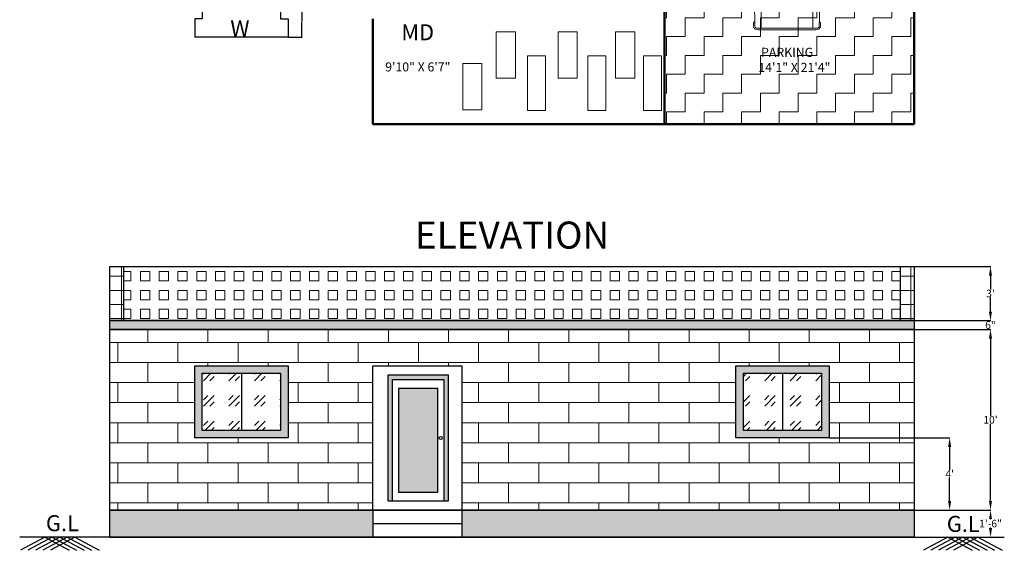
# Model space of a CAD drawing. Units: inches. Extents: x -105 to 1196, y -792 to 119.
# Tile 1 of 23: x -105 to 550, y -792 to -439. Entities that reach past the tile are written whole.
import ezdxf

# ---------------------------------------------------------------- set-up
doc = ezdxf.new("R2010")
doc.units = ezdxf.units.IN
doc.header["$MEASUREMENT"] = 0
for name, color, linetype, lineweight in [('A-ANNO-DIMS', 2, 'Continuous', 18), ('A-ANNO-TEXT', 7, 'Continuous', 25), ('A-AREA-IDEN', 7, 'Continuous', 25), ('A-DOOR', 4, 'Continuous', 25), ('A-ELEV', 6, 'Continuous', 25), ('A-ELEV-PATT', 8, 'Continuous', 13), ('A-EQPM', 8, 'Continuous', 18), ('A-FLOR-PATT', 252, 'Continuous', 13), ('A-GLAZ', 4, 'Continuous', 25), ('A-WALL', 3, 'Continuous', 50)]:
    doc.layers.add(name, color=color, linetype=linetype, lineweight=lineweight)
doc.styles.get("Standard").update_dxf_attribs({"font": 'arial.ttf'})
doc.dimstyles.get("Standard").update_dxf_attribs({"dimtxt": 0.18, "dimasz": 0.18, "dimexe": 0.18, "dimexo": 0.0625, "dimgap": 0.09, "dimtad": 0, "dimtih": 1, "dimtoh": 1, "dimdec": 1, "dimzin": 0, "dimdsep": 46, "dimlunit": 4, "dimtxsty": 'Standard', "dimcen": 0.09, "dimadec": 0, "dimazin": 0, "dimtfac": 1, "dimtdec": 1, "dimtofl": 0, "dimtmove": 0, "dimatfit": 3, "dimfxl": 1, "dimtolj": 1, "dimtzin": 0, "dimarcsym": 0})

# ---------------------------------------------------------------- blocks, each defined once
blk = doc.blocks.new('*U19')
for p, q in [((21.1, 37.4), (21.1, 36.8)), ((46.6, 38.9), (22.4, 38.9)), ((47.8, 37.4), (47.8, 37.4)), ((88, 31.9), (74.8, 35.9)), ((134.3, 35.6), (119.3, 31.8)), ((135.5, 37.1), (135.5, 37.4)), ((136.7, 38.9), (160.9, 38.9)), ((162.1, 37.4), (162.1, 36.8)), ((186.5, -33.5), (186.5, 33.5)), ((70, 31.5), (86.4, 29.4)), ((138.4, 29.4), (157.2, 29.4)), ((164.5, 26.4), (164.5, -26.4)), ((186.5, 29.4), (167, 29.4)), ((188.4, -32.8), (188.4, 32.8)), ((32.3, 11.6), (36.1, 17.2)), ((36.1, 17.2), (50.9, 17.2)), ((3.3, 6.1), (0.1, 0.4)), ((29.8, 9.5), (51.7, 9.5)), ((32.1, 9.5), (32.1, 11.2)), ((58.9, -10.8), (58.9, 10.8)), ((66.6, -10.5), (66.6, 10.5)), ((82.7, 8.5), (82.7, -8.5)), ((186.5, -10.5), (186.5, 10.5)), ((0, 0), (51.7, 0)), ((0.1, -0.4), (3.3, -6.1)), ((29.8, -9.5), (51.7, -9.5)), ((32.1, -9.5), (32.1, -11.2)), ((32.3, -11.6), (36.1, -17.2)), ((36.1, -17.2), (50.9, -17.2)), ((86.4, -29.4), (70, -31.5)), ((88, -31.9), (74.8, -35.9)), ((134.3, -35.6), (119.3, -31.8)), ((157.2, -29.4), (138.4, -29.4)), ((167, -29.4), (186.5, -29.4)), ((21.1, -37.4), (21.1, -36.8)), ((46.6, -38.9), (22.4, -38.9)), ((47.8, -37.4), (47.8, -37.4)), ((135.5, -37.1), (135.5, -37.4)), ((136.7, -38.9), (160.9, -38.9)), ((162.1, -37.4), (162.1, -36.8))]:
    blk.add_line(p, q)
for centre, major_axis, ratio, start_param, end_param in [((266, -27.5), (0, 313.3), 0.842304, 1.367076, 1.39176), ((41.2, -490.9), (0, 528.2), 0.842304, 0.00281, 0.075598), ((22.4, 37.4), (0, -1.48), 0.842304, 3.141593, 4.712389), ((64.5, -10555.6), (0, 10593), 0.842304, -0.013397, 0.002797), ((46.6, 37.4), (0, 1.48), 0.842304, -1.570796, 0), ((64.5, -10555.6), (0, -10591.5), 0.842304, 3.133765, 3.140441), ((136.7, 37.4), (0, -1.48), 0.842304, 3.141593, 4.712389), ((160.9, 37.4), (0, 1.48), 0.842304, -1.570796, 0), ((180.6, 35.8), (0, 2.22), 0.842304, -0.013017, 1.249894), ((64.5, -10556.4), (0, 10595.3), 0.842304, -0.013397, -0.013017), ((184, 32.8), (0, -5.25), 0.842304, 1.570796, 3.128196), ((184, 33.5), (0, -2.96), 0.842304, 1.570796, 3.128196), ((259.2, -27.5), (0, -305.3), 0.842304, 4.528606, 4.561838), ((37.5, -594), (0, -623.3), 0.842304, 3.096046, 3.200911), ((134.4, 5.4), (0, -89.8), 0.842304, 4.449482, 4.652344), ((135.3, 5.4), (0, 81.8), 0.842304, 1.245306, 1.50788), ((149.6, 2.8), (0, -79.6), 0.842304, 4.372215, 4.640744), ((95.8, -3666.4), (0, -3698.2), 0.842304, 3.134049, 3.144098), ((17.1, 0), (0, 147), 0.842304, 4.511394, 4.913384), ((35.9, 0), (0, 147), 0.842304, 4.511394, 4.913384), ((167, 26.4), (0, 2.96), 0.842304, 0, 1.570796), ((-204.5, 52.4), (0, -251), 0.842304, 1.385369, 1.434372), ((32.7, 11.2), (0, 0.74), 0.842304, 0.879714, 1.570796), ((13, 17), (0, 27.4), 0.842304, 4.435146, 4.718221), ((14.2, 17), (0, 27.4), 0.842304, 4.435146, 4.718221), ((50.8, 13.3), (6.34, -0.36), 0.603834, -1.395552, 1.581315), ((0.6, 0), (0, -0.74), 0.842304, 4.131459, 5.293319), ((29.8, -46.7), (0, 56.2), 0.842304, 0, 0.590319), ((-204.5, -52.4), (0, 251), 0.842304, -1.434372, -1.385369), ((29.8, 46.7), (0, 56.2), 0.842304, 2.551274, 3.141593), ((32.7, -11.2), (0, -0.74), 0.842304, 4.712389, 5.403472), ((13, -17), (0, -27.4), 0.842304, 1.564964, 1.848039), ((14.2, -17), (0, -27.4), 0.842304, 1.564964, 1.848039), ((134.4, -5.4), (0, -89.8), 0.842304, -1.510751, -1.307889), ((135.3, -5.4), (0, -81.8), 0.842304, -1.50788, -1.245306), ((149.6, -2.8), (0, -79.6), 0.842304, -1.499151, -1.230623), ((259.2, 27.5), (0, 305.3), 0.842304, 1.721348, 1.754579), ((266, 27.5), (0, 313.3), 0.842304, 1.749832, 1.774517), ((37.5, 594), (0, -623.3), 0.842304, -0.059319, 0.045547), ((95.8, 3666.4), (0, -3698.2), 0.842304, -0.002505, 0.007544), ((167, -26.4), (0, -2.96), 0.842304, 4.712389, 6.283185), ((184, -32.8), (0, -5.25), 0.842304, 0.013397, 1.570796), ((41.2, 490.9), (0, -528.2), 0.842304, -0.075598, -0.00281), ((22.4, -37.4), (0, 1.48), 0.842304, 1.570796, 3.141593), ((64.5, 10555.6), (0, 10593), 0.842304, 3.138796, 3.15499), ((46.6, -37.4), (0, -1.48), 0.842304, 0, 1.570796), ((64.5, 10555.6), (0, -10591.5), 0.842304, 0.001152, 0.007828), ((136.7, -37.4), (0, -1.48), 0.842304, -1.570796, 0), ((160.9, -37.4), (0, 1.48), 0.842304, 3.141593, 4.712389), ((180.6, -35.8), (0, -2.22), 0.842304, -1.249894, 0.013017), ((64.5, 10556.4), (0, 10595.3), 0.842304, 3.15461, 3.15499), ((184, -33.5), (0, 2.96), 0.842304, 3.15499, 4.712389)]:
    blk.add_ellipse(centre, major_axis=major_axis, ratio=ratio, start_param=start_param, end_param=end_param)
at = {"extrusion": (0, 0, -1)}
blk.add_ellipse((50.8, -13.3), major_axis=(6.34, 0.36), ratio=0.603834, start_param=-1.395552, end_param=1.581315, dxfattribs=at)
blk = doc.blocks.new('*U33')
blk.add_lwpolyline([(3.12, 0.01), (0.12, 0.01), (0.12, 84.01), (40.12, 84.01), (40.12, 0.01), (37.12, 0.01)])
for points in [[(37.12, 80.99), (37.12, 0.01), (3.12, 0.01), (3.12, 80.99)], [(33.12, 6.01), (33.12, 74.99), (7.12, 74.99), (7.12, 6.01)]]:
    blk.add_lwpolyline(points, close=True)
blk.add_circle((35.12, 42.01), 1)
blk = doc.blocks.new('*D35')
at = {"layer": 'A-ANNO-DIMS', "color": 0, "lineweight": -2, "transparency": 16777216}
for p, q in [((489.81, -764.85), (540.76, -764.85)), ((489.81, -782.85), (540.76, -782.85))]:
    blk.add_line(p, q, dxfattribs=at)
at = {"layer": 'A-ANNO-DIMS', "color": 0, "lineweight": 5, "transparency": 16777216}
for p, q in [((540.58, -770.85), (540.58, -771.21)), ((540.58, -776.85), (540.58, -776.49))]:
    blk.add_line(p, q, dxfattribs=at)
at = {"layer": 'A-ANNO-DIMS', "color": 0, "transparency": 16777216}
for points in [[(539.58, -770.85), (541.58, -770.85), (540.58, -764.85)], [(539.58, -776.85), (541.58, -776.85), (540.58, -782.85)]]:
    blk.add_solid(points, dxfattribs=at)
at = {"layer": 'Defpoints', "color": 0, "transparency": 16777216}
for p in [(489.74, -764.85), (540.58, -764.85), (489.74, -782.85)]:
    blk.add_point(p, dxfattribs=at)
at = {"layer": 'A-ANNO-DIMS', "color": 0, "transparency": 16777216, "insert": (540.58, -773.85), "char_height": 5, "attachment_point": 5}
blk.add_mtext('\\A1;1\'-6"', dxfattribs=at)
blk = doc.blocks.new('*D36')
at = {"layer": 'A-ANNO-DIMS', "color": 0, "lineweight": -2, "transparency": 16777216}
for p, q in [((489.81, -644.85), (540.73, -644.85)), ((540.55, -650.85), (540.55, -702.21)), ((540.55, -758.85), (540.55, -707.49)), ((489.81, -764.85), (540.73, -764.85))]:
    blk.add_line(p, q, dxfattribs=at)
at = {"layer": 'A-ANNO-DIMS', "color": 0, "transparency": 16777216}
for points in [[(539.55, -650.85), (541.55, -650.85), (540.55, -644.85)], [(539.55, -758.85), (541.55, -758.85), (540.55, -764.85)]]:
    blk.add_solid(points, dxfattribs=at)
at = {"layer": 'Defpoints', "color": 0, "transparency": 16777216}
for p in [(489.74, -644.85), (540.55, -644.85), (489.74, -764.85)]:
    blk.add_point(p, dxfattribs=at)
at = {"layer": 'A-ANNO-DIMS', "color": 0, "transparency": 16777216, "insert": (540.55, -704.85), "char_height": 5, "attachment_point": 5}
blk.add_mtext("\\A1;10'", dxfattribs=at)
blk = doc.blocks.new('*D37')
at = {"layer": 'A-ANNO-DIMS', "color": 0, "lineweight": -2, "transparency": 16777216}
for p, q in [((433.31, -716.85), (513.56, -716.85)), ((513.38, -722.85), (513.38, -738.26)), ((513.38, -758.85), (513.38, -743.44)), ((489.81, -764.85), (513.56, -764.85))]:
    blk.add_line(p, q, dxfattribs=at)
at = {"layer": 'A-ANNO-DIMS', "color": 0, "transparency": 16777216}
for points in [[(512.38, -722.85), (514.38, -722.85), (513.38, -716.85)], [(512.38, -758.85), (514.38, -758.85), (513.38, -764.85)]]:
    blk.add_solid(points, dxfattribs=at)
at = {"layer": 'Defpoints', "color": 0, "transparency": 16777216}
for p in [(433.24, -716.85), (489.74, -764.85), (513.38, -764.85)]:
    blk.add_point(p, dxfattribs=at)
at = {"layer": 'A-ANNO-DIMS', "color": 0, "transparency": 16777216, "insert": (513.38, -740.85), "char_height": 5, "attachment_point": 5}
blk.add_mtext("\\A1;4'", dxfattribs=at)
blk = doc.blocks.new('*D38')
at = {"layer": 'A-ANNO-DIMS', "color": 0, "lineweight": -2, "transparency": 16777216}
for p, q in [((540.53, -632.85), (540.53, -626.85)), ((489.81, -638.85), (540.71, -638.85)), ((489.81, -644.85), (540.71, -644.85)), ((540.53, -650.85), (540.53, -656.85))]:
    blk.add_line(p, q, dxfattribs=at)
at = {"layer": 'A-ANNO-DIMS', "color": 0, "transparency": 16777216}
for points in [[(539.53, -632.85), (541.53, -632.85), (540.53, -638.85)], [(539.53, -650.85), (541.53, -650.85), (540.53, -644.85)]]:
    blk.add_solid(points, dxfattribs=at)
at = {"layer": 'Defpoints', "color": 0, "transparency": 16777216}
for p in [(489.74, -638.85), (540.53, -638.85), (489.74, -644.85)]:
    blk.add_point(p, dxfattribs=at)
at = {"layer": 'A-ANNO-DIMS', "color": 0, "transparency": 16777216, "insert": (540.53, -641.85), "char_height": 5, "attachment_point": 5}
blk.add_mtext('\\A1;6"', dxfattribs=at)
blk = doc.blocks.new('*D39')
at = {"layer": 'A-ANNO-DIMS', "color": 0, "lineweight": -2, "transparency": 16777216}
for p, q in [((489.81, -602.85), (540.73, -602.85)), ((540.55, -608.85), (540.55, -618.2)), ((540.55, -632.85), (540.55, -623.49)), ((489.81, -638.85), (540.73, -638.85))]:
    blk.add_line(p, q, dxfattribs=at)
at = {"layer": 'A-ANNO-DIMS', "color": 0, "transparency": 16777216}
for points in [[(539.55, -608.85), (541.55, -608.85), (540.55, -602.85)], [(539.55, -632.85), (541.55, -632.85), (540.55, -638.85)]]:
    blk.add_solid(points, dxfattribs=at)
at = {"layer": 'Defpoints', "color": 0, "transparency": 16777216}
for p in [(489.74, -602.85), (489.74, -638.85), (540.55, -638.85)]:
    blk.add_point(p, dxfattribs=at)
at = {"layer": 'A-ANNO-DIMS', "color": 0, "transparency": 16777216, "insert": (540.55, -620.85), "char_height": 5, "attachment_point": 5}
blk.add_mtext("\\A1;3'", dxfattribs=at)
blk = doc.blocks.new('WIN-1200')
at = {"ltscale": 2}
for p, q in [((12, 62), (0, 62)), ((0, 0), (0, 62)), ((12, 57), (12, 62)), ((12, 5), (12, 0)), ((12, 0), (0, 0))]:
    blk.add_line(p, q, dxfattribs=at)
for p, q in [((21, 57), (12, 57)), ((21, 5), (12, 5))]:
    blk.add_line(p, q)
blk = doc.blocks.new('*D56')
at = {"layer": 'A-ANNO-DIMS', "color": 0, "lineweight": -2, "transparency": 16777216}
for p, q in [((73.31, -429.23), (82.72, -429.23)), ((82.54, -429.41), (82.54, -439.55)), ((82.54, -450.05), (82.54, -439.91)), ((73.31, -450.23), (82.72, -450.23))]:
    blk.add_line(p, q, dxfattribs=at)
at = {"layer": 'A-ANNO-DIMS', "color": 0, "transparency": 16777216}
for points in [[(82.51, -429.41), (82.57, -429.41), (82.54, -429.23)], [(82.51, -450.05), (82.57, -450.05), (82.54, -450.23)]]:
    blk.add_solid(points, dxfattribs=at)
at = {"layer": 'Defpoints', "color": 0, "transparency": 16777216}
for p in [(73.24, -429.23), (82.54, -429.23), (73.24, -450.23)]:
    blk.add_point(p, dxfattribs=at)
at = {"layer": 'A-ANNO-DIMS', "color": 0, "transparency": 16777216, "insert": (82.54, -439.73), "char_height": 0.18, "attachment_point": 5}
blk.add_mtext('\\A1;1\'-9" TYP.', dxfattribs=at)

msp = doc.modelspace()

# ---------------------------------------------------------------- hatches: boundary and pattern name
at = {"layer": 'A-ELEV-PATT'}
h = msp.add_hatch(dxfattribs=at)
h.set_pattern_fill('NET', color=256, scale=75)
h.paths.add_polyline_path([(-36.26, -602.85), (-45.26, -602.85), (-45.26, -638.85), (-36.26, -638.85)])
h.paths.add_polyline_path([(489.74, -602.85), (480.74, -602.85), (480.74, -638.85), (489.74, -638.85)])
h = msp.add_hatch(dxfattribs=at)
h.set_pattern_fill('SQUARE', color=256, scale=50)
h.paths.add_polyline_path([(480.74, -602.85), (-36.26, -602.85), (-36.26, -638.85), (480.74, -638.85)])
h = msp.add_hatch(color=256, dxfattribs=at)
h.dxf.hatch_style = 1
h.paths.add_polyline_path([(489.74, -638.85), (-45.26, -638.85), (-45.26, -644.85), (489.74, -644.85)])
h.paths.add_polyline_path([(73.24, -668.85), (11.24, -668.85), (11.24, -716.85), (73.24, -716.85)])
h.paths.add_polyline_path([(68.24, -673.85), (68.24, -711.85), (16.24, -711.85), (16.24, -673.85)], flags=16)
h.paths.add_polyline_path([(433.24, -668.85), (371.24, -668.85), (371.24, -716.85), (433.24, -716.85)])
h.paths.add_polyline_path([(428.24, -673.85), (428.24, -711.85), (376.24, -711.85), (376.24, -673.85)], flags=16)
h = msp.add_hatch(dxfattribs=at)
h.set_pattern_fill('AR-BRSTD', color=256, scale=5)
h.paths.add_polyline_path([(489.74, -644.85), (-45.26, -644.85), (-45.26, -764.85), (129.74, -764.85), (129.74, -668.85), (188.8, -668.85), (188.8, -764.85), (489.74, -764.85)])
h.paths.add_polyline_path([(371.24, -668.85), (433.24, -668.85), (433.24, -716.85), (371.24, -716.85)], flags=16)
h.paths.add_polyline_path([(376.24, -673.85), (428.24, -673.85), (428.24, -711.85), (376.24, -711.85)], flags=0)
h.paths.add_polyline_path([(73.24, -716.85), (11.24, -716.85), (11.24, -668.85), (73.24, -668.85)], flags=16)
h.paths.add_polyline_path([(68.24, -711.85), (16.24, -711.85), (16.24, -673.85), (68.24, -673.85)], flags=0)
h = msp.add_hatch(dxfattribs=at)
h.set_pattern_fill('GOST_GLASS', color=256, scale=2)
h.set_pattern_definition([(45, (0, 0), (16.97056, -2e-15), [10, -14]), (45, (4.243, 0), (16.97056, -2e-15), [4, -20]), (45, (0, 4.243), (16.97056, -2e-15), [4, -20])])
h.paths.add_polyline_path([(42.24, -673.85), (16.24, -673.85), (16.24, -711.85), (42.24, -711.85)])
h.paths.add_polyline_path([(68.24, -673.85), (42.24, -673.85), (42.24, -711.85), (68.24, -711.85)])
h.paths.add_polyline_path([(402.24, -673.85), (376.24, -673.85), (376.24, -711.85), (402.24, -711.85)])
h.paths.add_polyline_path([(428.24, -673.85), (402.24, -673.85), (402.24, -711.85), (428.24, -711.85)])
h = msp.add_hatch(color=256, dxfattribs=at)
h.dxf.hatch_style = 1
h.paths.add_polyline_path([(172.82, -683.92), (146.82, -683.92), (146.82, -752.9), (172.82, -752.9)], flags=17)
h.paths.add_polyline_path([(142.82, -677.92), (176.82, -677.92), (176.82, -758.9), (179.82, -758.9), (179.82, -674.9), (139.82, -674.9), (139.82, -758.9), (142.82, -758.9)])
h = msp.add_hatch(dxfattribs=at)
h.set_pattern_fill('AR-CONC', color=256, scale=2)
h.paths.add_polyline_path([(129.74, -764.85), (-45.26, -764.85), (-45.26, -782.85), (129.74, -782.85)])
h.paths.add_polyline_path([(489.74, -764.85), (188.8, -764.85), (188.8, -782.85), (489.74, -782.85)])
at = {"layer": 'A-FLOR-PATT'}
h = msp.add_hatch(dxfattribs=at)
h.set_pattern_fill('ZIGZAG', color=256, scale=100)
h.set_pattern_definition([(0, (0, 0), (12.5, 12.5), [12.5, -12.5]), (90, (12.5, 0), (-12.5, 12.5), [12.5, -12.5])])
h.paths.add_polyline_path([(489.74, -331.23), (323.74, -331.23), (323.74, -508.23), (489.74, -508.23)])
h.paths.add_polyline_path([(383.72, -476.81), (434.09, -476.81), (434.09, -454.42), (383.72, -454.42)], flags=24)

# ---------------------------------------------------------------- linework, layer by layer
at = {"layer": 'A-ELEV'}
for p, q in [((-45.26, -602.85), (489.74, -602.85)), ((-45.26, -638.85), (489.74, -638.85)), ((-45.26, -644.85), (489.74, -644.85)), ((42.24, -673.85), (42.24, -711.85)), ((402.24, -673.85), (402.24, -711.85)), ((-45.26, -764.85), (489.74, -764.85)), ((129.74, -764.85), (188.8, -764.85)), ((129.74, -764.85), (129.74, -782.85)), ((188.8, -764.85), (188.8, -782.85)), ((129.74, -773.85), (188.8, -773.85)), ((-45.26, -782.85), (-105.26, -782.85)), ((-88.58, -782.85), (-104.77, -791.63)), ((-83.58, -782.85), (-99.77, -791.63)), ((-78.58, -782.85), (-94.77, -791.63)), ((-73.58, -782.85), (-89.77, -791.63)), ((-88.58, -782.85), (-72.39, -791.63)), ((-68.58, -782.85), (-84.77, -791.63)), ((-83.58, -782.85), (-67.39, -791.63)), ((-78.58, -782.85), (-62.39, -791.63)), ((-73.58, -782.85), (-57.39, -791.63)), ((-68.58, -782.85), (-52.39, -791.63)), ((-45.26, -782.85), (489.74, -782.85)), ((489.74, -782.85), (549.74, -782.85)), ((512.12, -782.85), (495.93, -791.63)), ((517.12, -782.85), (500.93, -791.63)), ((522.12, -782.85), (505.93, -791.63)), ((527.12, -782.85), (510.93, -791.63)), ((512.12, -782.85), (528.31, -791.63)), ((532.12, -782.85), (515.93, -791.63)), ((517.12, -782.85), (533.31, -791.63)), ((522.12, -782.85), (538.31, -791.63)), ((527.12, -782.85), (543.31, -791.63)), ((532.12, -782.85), (548.31, -791.63))]:
    msp.add_line(p, q, dxfattribs=at)
for points in [[(-45.26, -602.85), (489.74, -602.85), (489.74, -638.85), (-45.26, -638.85)], [(-45.26, -602.85), (-36.26, -602.85), (-36.26, -638.85), (-45.26, -638.85)], [(480.74, -602.85), (489.74, -602.85), (489.74, -638.85), (480.74, -638.85)], [(-45.26, -638.85), (489.74, -638.85), (489.74, -644.85), (-45.26, -644.85)], [(-45.26, -644.85), (489.74, -644.85), (489.74, -764.85), (-45.26, -764.85)], [(11.24, -668.85), (73.24, -668.85), (73.24, -716.85), (11.24, -716.85)], [(16.24, -673.85), (68.24, -673.85), (68.24, -711.85), (16.24, -711.85)], [(129.74, -668.85), (188.8, -668.85), (188.8, -764.85), (129.74, -764.85)], [(371.24, -668.85), (433.24, -668.85), (433.24, -716.85), (371.24, -716.85)], [(376.24, -673.85), (428.24, -673.85), (428.24, -711.85), (376.24, -711.85)], [(-45.26, -764.85), (489.74, -764.85), (489.74, -782.85), (-45.26, -782.85)]]:
    msp.add_lwpolyline(points, close=True, dxfattribs=at)
at = {"layer": 'A-FLOR-PATT'}
for points in [[(211.78, -446.84), (224.55, -446.84), (224.55, -477.64), (211.78, -477.64)], [(252.86, -446.84), (265.63, -446.84), (265.63, -477.64), (252.86, -477.64)], [(291.14, -446.84), (303.91, -446.84), (303.91, -477.64), (291.14, -477.64)], [(232.62, -462.71), (244.46, -462.71), (244.46, -499.11), (232.62, -499.11)], [(272.76, -462.71), (284.6, -462.71), (284.6, -499.11), (272.76, -499.11)], [(309.83, -462.71), (321.67, -462.71), (321.67, -499.11), (309.83, -499.11)], [(189.48, -467.86), (202.25, -467.86), (202.25, -498.66), (189.48, -498.66)]]:
    msp.add_lwpolyline(points, close=True, dxfattribs=at)
at = {"layer": 'A-WALL'}
for p, q in [((489.74, -125.23), (489.74, -508.23)), ((323.74, -331.23), (323.74, -508.23)), ((129.74, -438.23), (129.74, -508.23)), ((129.74, -508.23), (489.74, -508.23))]:
    msp.add_line(p, q, dxfattribs=at)

# ---------------------------------------------------------------- block references
at = {"layer": 'A-DOOR'}
msp.add_blockref('*U33', (139.7, -758.91), dxfattribs=at)
at = {"layer": 'A-EQPM', "xscale": 0.5869636799172785, "yscale": 0.5869636799172785, "zscale": 0.5869636799172785, "rotation": 270}
msp.add_blockref('*U19', (405.22, -334.89), dxfattribs=at)
at = {"layer": 'A-GLAZ', "rotation": 90.00000000000006}
msp.add_blockref('WIN-1200', (73.24, -450.23), dxfattribs=at)

# ---------------------------------------------------------------- texts
at = {"layer": 'A-ANNO-TEXT'}
for s, height, p in [('W', 10.64, (34.87, -449.82)), ('MD', 10.636, (148.63, -452.39)), ('ELEVATION', 18, (157.7, -590.98)), ('G.L', 10.636, (-87.8, -778.91)), ('G.L', 10.636, (511.49, -779.38))]:
    msp.add_text(s, height=height, dxfattribs=at).set_placement(p)
at = {"layer": 'A-AREA-IDEN', "char_height": 6, "attachment_point": 1}
for s, insert in [(' PARKING\\P14\'1" X 21\'4"', (386.13, -457.41)), (' \\P9\'10" X 6\'7"', (137.9, -467.12))]:
    msp.add_mtext_dynamic_manual_height_columns(s, width=59.5623, gutter_width=1, heights=[0], dxfattribs=dict(at, insert=insert))

# ---------------------------------------------------------------- dimensions: what is measured, and where the dimension line sits
at = {"layer": 'A-ANNO-DIMS'}
dim = msp.add_linear_dim(base=(82.54, -429.23), p1=(73.24, -450.23), p2=(73.24, -429.23), angle=90, text='<> TYP.', dimstyle='Standard', override={"dimdec": 1, "dimlfac": 1, "dimrnd": 0, "dimzin": 1, "dimdsep": 46, "dimlunit": 4, "dimfrac": 2}, dxfattribs=at)
dim.commit()
dim.dimension.update_dxf_attribs({"geometry": '*D56', "text_midpoint": (82.54, -439.73)})
for base, p1, p2, override, picture, middle in [((540.55, -638.85), (489.74, -602.85), (489.74, -638.85), {"dimtxt": 5, "dimasz": 6, "dimclrd": 0, "dimclre": 0, "dimclrt": 0}, '*D39', (540.55, -620.85)), ((540.53, -638.85), (489.74, -644.85), (489.74, -638.85), {"dimtxt": 5, "dimasz": 6, "dimclrd": 0, "dimclre": 0, "dimclrt": 0}, '*D38', (540.53, -641.85)), ((540.55, -644.85), (489.74, -764.85), (489.74, -644.85), {"dimtxt": 5, "dimasz": 6, "dimclrd": 0, "dimclre": 0, "dimclrt": 0}, '*D36', (540.55, -704.85)), ((513.38, -764.85), (433.24, -716.85), (489.74, -764.85), {"dimtxt": 5, "dimasz": 6, "dimclrd": 0, "dimclre": 0, "dimclrt": 0}, '*D37', (513.38, -740.85)), ((540.58, -764.85), (489.74, -782.85), (489.74, -764.85), {"dimtxt": 5, "dimasz": 6, "dimclrd": 0, "dimclre": 0, "dimclrt": 0, "dimlwd": 5}, '*D35', (540.58, -773.85))]:
    dim = msp.add_linear_dim(base=base, p1=p1, p2=p2, angle=90, dimstyle='Standard', override=override, dxfattribs=at)
    dim.commit()
    dim.dimension.update_dxf_attribs({"geometry": picture, "text_midpoint": middle})

doc.saveas('drawing.dxf')
